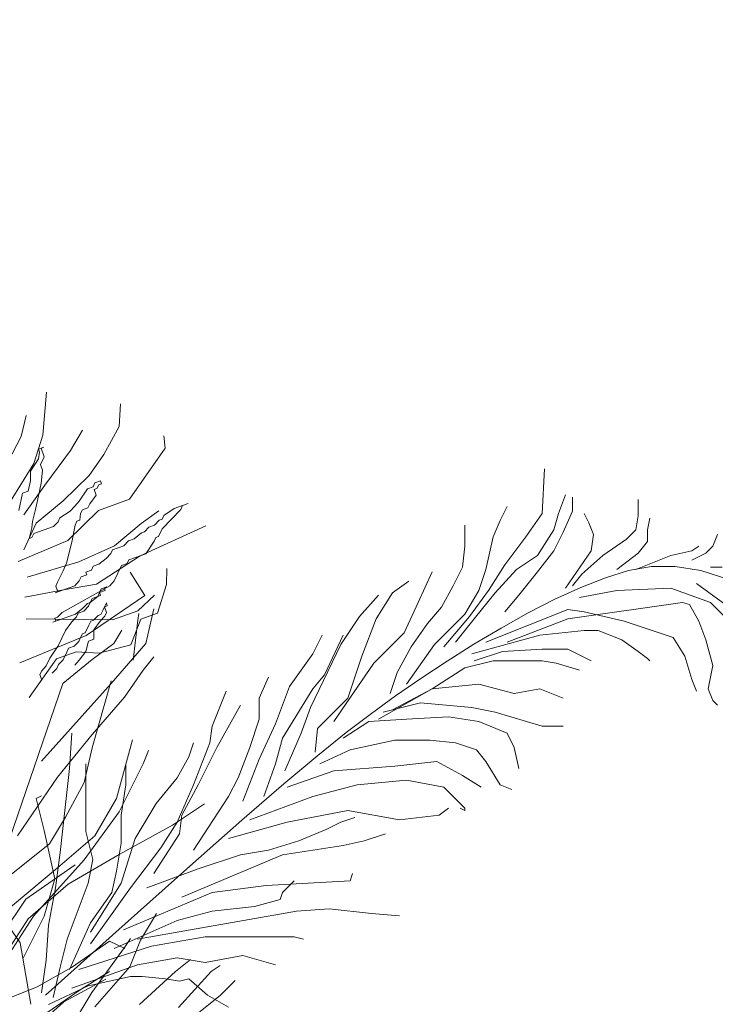
# Model space of a CAD drawing. Units: millimetres. Extents: x 595116 to 630915, y 909473 to 920225.
# Tile 89 of 134: x 629720.901 to 629727.558, y 919275.684 to 919285.103. Entities that reach past the tile are written whole.
import ezdxf

# ---------------------------------------------------------------- set-up
doc = ezdxf.new("R2010")
doc.units = ezdxf.units.MM
doc.layers.add('Dimension', color=3, linetype='Continuous', lineweight=18)
doc.layers.add('L-PLNT', color=85, linetype='Continuous', lineweight=13)
doc.styles.get("Standard").update_dxf_attribs({"font": 'arial.ttf'})
doc.dimstyles.new('ISO-25', dxfattribs={"dimtxt": 9, "dimasz": 6, "dimexe": 1.25, "dimexo": 0.625, "dimtad": 1, "dimlunit": 4, "dimtxsty": 'Standard', "dimcen": 2.5, "dimadec": 0, "dimazin": 0, "dimtfac": 1, "dimtmove": 0, "dimatfit": 3, "dimfxl": 1, "dimarcsym": 0})

# ---------------------------------------------------------------- blocks, each defined once
blk = doc.blocks.new('A$C4FB75ABC')
for p, q in [((2.8876, 3.7608), (2.897, 3.8696)), ((3.0823, 3.7823), (3.0858, 3.8403)), ((2.8322, 3.7571), (2.8454, 3.8105)), ((2.9584, 3.7215), (2.9885, 3.7729)), ((3.043, 3.7114), (3.0823, 3.7823)), ((2.7745, 3.6472), (2.8322, 3.7571)), ((2.8652, 3.6879), (2.8876, 3.7608)), ((3.1994, 3.7272), (3.1962, 3.7584)), ((2.8907, 3.7295), (2.8764, 3.7244)), ((2.8764, 3.7244), (2.8789, 3.7172)), ((2.8789, 3.7172), (2.8769, 3.7003)), ((2.8835, 3.727), (2.8907, 3.7295)), ((2.8913, 3.7054), (2.8835, 3.727)), ((2.893, 3.6331), (2.9584, 3.7215)), ((3.1085, 3.5972), (3.1994, 3.7272)), ((2.8769, 3.7003), (2.856, 3.6684)), ((2.8821, 3.6859), (2.8913, 3.7054)), ((3.0058, 3.6575), (3.043, 3.7114)), ((2.7932, 3.5729), (2.8652, 3.6879)), ((2.856, 3.6684), (2.8566, 3.6443)), ((2.8873, 3.6716), (2.8821, 3.6859)), ((2.8833, 3.6377), (2.8873, 3.6716)), ((4.1608, 3.5609), (4.1668, 3.6742)), ((2.8566, 3.6443), (2.85, 3.6176)), ((2.9398, 3.5932), (3.0058, 3.6575)), ((3.035, 3.6437), (3.0207, 3.6385)), ((3.0376, 3.6365), (3.035, 3.6437)), ((2.85, 3.6176), (2.8356, 3.6125)), ((2.8394, 3.5571), (2.893, 3.6331)), ((2.8746, 3.5941), (2.8833, 3.6377)), ((3.0017, 3.6236), (2.9808, 3.5918)), ((3.0161, 3.6288), (3.0017, 3.6236)), ((3.0207, 3.6385), (3.0161, 3.6288)), ((3.0187, 3.6216), (3.0258, 3.6242)), ((3.0238, 3.6072), (3.0187, 3.6216)), ((3.0258, 3.6242), (3.0304, 3.6339)), ((3.0304, 3.6339), (3.0376, 3.6365)), ((2.8356, 3.6125), (2.827, 3.5688)), ((2.868, 3.5674), (2.8746, 3.5941)), ((2.8712, 3.5361), (2.9398, 3.5932)), ((2.9808, 3.5918), (2.969, 3.5794)), ((3.0075, 3.5852), (3.0238, 3.6072)), ((3.0296, 3.5688), (3.1085, 3.5972)), ((4.2026, 3.5609), (4.2205, 3.6086)), ((4.2384, 3.5668), (4.2384, 3.6026)), ((4.4054, 3.5549), (4.4054, 3.5967)), ((2.8614, 3.5407), (2.868, 3.5674)), ((2.9573, 3.5671), (2.9312, 3.5496)), ((2.9518, 3.4922), (3.0296, 3.5688)), ((2.969, 3.5794), (2.9573, 3.5671)), ((2.984, 3.5605), (2.9885, 3.5702)), ((2.9885, 3.5702), (3.0029, 3.5754)), ((3.0029, 3.5754), (3.0075, 3.5852)), ((3.1389, 3.5352), (3.1839, 3.5676)), ((3.2224, 3.5733), (3.1962, 3.5558)), ((3.2158, 3.5466), (3.2393, 3.5713)), ((3.2582, 3.5862), (3.2224, 3.5733)), ((3.2393, 3.5713), (3.2439, 3.5811)), ((3.2439, 3.5811), (3.2582, 3.5862)), ((4.0535, 3.543), (4.0714, 3.5788)), ((4.2145, 3.5132), (4.2384, 3.5668)), ((2.8594, 3.5238), (2.8614, 3.5407)), ((2.9266, 3.5398), (2.9148, 3.5275)), ((2.9312, 3.5496), (2.9266, 3.5398)), ((2.9702, 3.5312), (2.9748, 3.541)), ((2.9748, 3.541), (2.9819, 3.5435)), ((2.9819, 3.5435), (2.984, 3.5605)), ((3.1845, 3.5435), (3.1727, 3.5311)), ((3.1917, 3.5461), (3.1845, 3.5435)), ((3.1962, 3.5558), (3.1917, 3.5461)), ((3.1922, 3.522), (3.2158, 3.5466)), ((4.0356, 3.5013), (4.0535, 3.543)), ((4.1191, 3.5013), (4.1608, 3.5609)), ((4.1907, 3.5192), (4.2026, 3.5609)), ((4.2801, 3.537), (4.2682, 3.5609)), ((4.3994, 3.5192), (4.4054, 3.5549)), ((4.4293, 3.5192), (4.4352, 3.549)), ((2.8391, 3.4678), (2.8712, 3.5361)), ((2.8528, 3.4971), (2.8594, 3.5238)), ((2.9148, 3.5275), (2.8646, 3.5094)), ((2.9616, 3.4876), (2.9702, 3.5312)), ((3.0703, 3.4781), (3.1389, 3.5352)), ((3.136, 3.4531), (3.303, 3.5294)), ((3.1466, 3.5136), (3.1394, 3.5111)), ((3.1584, 3.526), (3.1466, 3.5136)), ((3.1727, 3.5311), (3.1584, 3.526)), ((3.1831, 3.5024), (3.1922, 3.522)), ((3.964, 3.4774), (3.964, 3.5311)), ((4.1489, 3.4536), (4.1907, 3.5192)), ((4.2921, 3.5072), (4.2801, 3.537)), ((4.3756, 3.4953), (4.3994, 3.5192)), ((4.4293, 3.4893), (4.4293, 3.5192)), ((2.8253, 3.4385), (2.9518, 3.4922)), ((2.86, 3.4997), (2.8528, 3.4971)), ((2.8646, 3.5094), (2.86, 3.4997)), ((3.1062, 3.491), (3.0944, 3.4786)), ((3.1205, 3.4961), (3.1062, 3.491)), ((3.1394, 3.5111), (3.1205, 3.4961)), ((3.1503, 3.4583), (3.1713, 3.4901)), ((3.1713, 3.4901), (3.1759, 3.4999)), ((3.1759, 3.4999), (3.1831, 3.5024)), ((4.0177, 3.4178), (4.0356, 3.5013)), ((4.0654, 3.4297), (4.1191, 3.5013)), ((4.1907, 3.4655), (4.2145, 3.5132)), ((4.2861, 3.4655), (4.2921, 3.5072)), ((4.3159, 3.4536), (4.3756, 3.4953)), ((4.4054, 3.4595), (4.4293, 3.4893)), ((4.5963, 3.4774), (4.6082, 3.5072)), ((2.9484, 3.4342), (2.9616, 3.4876)), ((2.9797, 3.4374), (3.0703, 3.4781)), ((3.0657, 3.4683), (3.0611, 3.4586)), ((3.0944, 3.4786), (3.0657, 3.4683)), ((3.958, 3.4238), (3.964, 3.4774)), ((4.1489, 3.4118), (4.1907, 3.4655)), ((4.2205, 3.3701), (4.2861, 3.4655)), ((4.4889, 3.4536), (4.5426, 3.4655)), ((4.5426, 3.4655), (4.5605, 3.4774)), ((4.5784, 3.4595), (4.5963, 3.4774)), ((3.0244, 3.3805), (3.136, 3.4531)), ((3.0494, 3.4462), (3.0304, 3.4313)), ((3.0611, 3.4586), (3.0494, 3.4462)), ((3.1027, 3.433), (3.1073, 3.4428)), ((3.1073, 3.4428), (3.1503, 3.4583)), ((4.0952, 3.4178), (4.1489, 3.4536)), ((4.2622, 3.4059), (4.3159, 3.4536)), ((4.3517, 3.4178), (4.4054, 3.4595)), ((4.3994, 3.4178), (4.4889, 3.4536)), ((4.5426, 3.4416), (4.5784, 3.4595)), ((2.848, 3.3981), (2.9797, 3.4374)), ((2.9254, 3.3854), (2.9392, 3.4147)), ((2.9392, 3.4147), (2.9484, 3.4342)), ((3.0115, 3.4164), (2.9972, 3.4112)), ((3.0161, 3.4262), (3.0115, 3.4164)), ((3.0304, 3.4313), (3.0161, 3.4262)), ((3.07, 3.3888), (3.0884, 3.4279)), ((3.0884, 3.4279), (3.1027, 3.433)), ((3.2028, 3.3799), (3.2043, 3.4209)), ((3.9342, 3.3761), (3.958, 3.4238)), ((3.9998, 3.3641), (4.0177, 3.4178)), ((4.0237, 3.3641), (4.0654, 3.4297)), ((4.0415, 3.3582), (4.0952, 3.4178)), ((4.322, 3.3969), (4.3813, 3.4152)), ((4.3813, 3.4152), (4.4396, 3.4254)), ((4.4396, 3.4254), (4.5001, 3.426)), ((4.5001, 3.426), (4.5657, 3.4153)), ((4.5657, 3.4153), (4.6395, 3.3917)), ((4.5903, 3.4238), (4.6201, 3.4238)), ((2.9808, 3.3891), (2.969, 3.3768)), ((2.9854, 3.3989), (2.9808, 3.3891)), ((2.9997, 3.4041), (2.9854, 3.3989)), ((2.9972, 3.4112), (2.9997, 3.4041)), ((3.0583, 3.3765), (3.07, 3.3888)), ((3.1481, 3.3521), (3.1105, 3.4115)), ((3.7791, 3.3582), (3.8208, 3.388)), ((3.8447, 3.3343), (3.8805, 3.4118)), ((4.1012, 3.3522), (4.1489, 3.4118)), ((4.2384, 3.3761), (4.2622, 3.4059)), ((4.2593, 3.3722), (4.322, 3.3969)), ((2.8419, 3.3473), (2.9403, 3.3665)), ((2.969, 3.3768), (2.9188, 3.3587)), ((2.9208, 3.3757), (2.9254, 3.3854)), ((2.926, 3.3613), (2.9208, 3.3757)), ((2.9369, 3.3085), (3.0583, 3.3765)), ((2.9403, 3.3665), (3.0244, 3.3805)), ((3.0367, 3.3687), (3.0322, 3.359)), ((3.0322, 3.359), (3.0465, 3.3642)), ((3.0511, 3.3739), (3.0367, 3.3687)), ((3.0439, 3.3713), (3.0511, 3.3739)), ((3.0465, 3.3642), (3.0439, 3.3713)), ((3.1805, 3.307), (3.2028, 3.3799)), ((3.9044, 3.3224), (3.9342, 3.3761)), ((3.964, 3.3045), (3.9998, 3.3641)), ((3.9759, 3.2986), (4.0237, 3.3641)), ((4.1935, 3.342), (4.2593, 3.3722)), ((4.2563, 3.3463), (4.3517, 3.3641)), ((4.3517, 3.3641), (4.4889, 3.3701)), ((4.4889, 3.3701), (4.5903, 3.3343)), ((4.5545, 3.382), (4.6858, 3.2866)), ((2.9188, 3.3587), (2.926, 3.3613)), ((2.9986, 3.2497), (3.1481, 3.3521)), ((3.0276, 3.3492), (3.0086, 3.3343)), ((3.0086, 3.3343), (3.0132, 3.3441)), ((3.0132, 3.3441), (3.0347, 3.3518)), ((3.0322, 3.359), (3.0276, 3.3492)), ((3.0347, 3.3518), (3.0322, 3.359)), ((3.1297, 3.313), (3.1722, 3.3526)), ((3.6956, 3.2986), (3.7433, 3.3522)), ((3.7373, 3.2926), (3.7791, 3.3582)), ((3.9879, 3.2926), (4.0415, 3.3582)), ((4.0654, 3.3105), (4.1012, 3.3522)), ((4.1256, 3.3072), (4.1935, 3.342)), ((2.9897, 3.3194), (2.9708, 3.3045)), ((3.0015, 3.3317), (2.9897, 3.3194)), ((2.9923, 3.3122), (3.004, 3.3246)), ((3.0086, 3.3343), (3.0015, 3.3317)), ((3.004, 3.3246), (3.0086, 3.3343)), ((3.0359, 3.3036), (3.0405, 3.3134)), ((3.0405, 3.3134), (3.0451, 3.3231)), ((3.0497, 3.3329), (3.0451, 3.3231)), ((3.0451, 3.3231), (3.0522, 3.3257)), ((3.0451, 3.3231), (3.0502, 3.3088)), ((3.0522, 3.3257), (3.0497, 3.3329)), ((3.0651, 3.2898), (3.1297, 3.313)), ((3.1501, 3.2292), (3.1706, 3.3178)), ((3.8089, 3.2568), (3.8447, 3.3343)), ((3.8686, 3.2807), (3.9044, 3.3224)), ((4.0177, 3.233), (4.2265, 3.3164)), ((4.2265, 3.2926), (4.5187, 3.3343)), ((4.2265, 3.3164), (4.2682, 3.3105)), ((4.5187, 3.3343), (4.5366, 3.3284)), ((4.5366, 3.3284), (4.5605, 3.2866)), ((4.5903, 3.3343), (4.644, 3.2807)), ((2.8457, 3.2919), (3.0651, 3.2898)), ((2.9708, 3.3045), (2.9134, 3.2838)), ((2.918, 3.2936), (2.9251, 3.2962)), ((2.9206, 3.2864), (2.918, 3.2936)), ((2.9251, 3.2962), (2.9369, 3.3085)), ((2.9616, 3.285), (2.9733, 3.2973)), ((2.9733, 3.2973), (2.9779, 3.3071)), ((2.9779, 3.3071), (2.9923, 3.3122)), ((3.0098, 3.2861), (3.0169, 3.2887)), ((3.0169, 3.2887), (3.0287, 3.301)), ((3.0287, 3.301), (3.0359, 3.3036)), ((3.0456, 3.299), (3.0339, 3.2867)), ((3.0502, 3.3088), (3.0456, 3.299)), ((3.1125, 3.2258), (3.1374, 3.2915)), ((3.1182, 3.1873), (3.1303, 3.2889)), ((3.1303, 3.2889), (3.1323, 3.3059)), ((3.1374, 3.2915), (3.1805, 3.307)), ((3.6479, 3.227), (3.6956, 3.2986)), ((3.7015, 3.1972), (3.7373, 3.2926)), ((3.8865, 3.227), (3.964, 3.3045)), ((3.9103, 3.2211), (3.9759, 3.2986)), ((3.9401, 3.233), (3.9879, 3.2926)), ((4.0565, 3.2687), (4.1256, 3.3072)), ((4.0714, 3.233), (4.2265, 3.2926)), ((4.2682, 3.3105), (4.3696, 3.2866)), ((2.9134, 3.2838), (2.9206, 3.2864)), ((2.936, 3.2434), (2.9452, 3.2629)), ((2.9452, 3.2629), (2.9616, 3.285)), ((2.996, 3.2568), (3.0052, 3.2763)), ((3.0052, 3.2763), (3.0098, 3.2861)), ((3.0339, 3.2867), (3.0175, 3.2646)), ((3.0175, 3.2646), (3.0181, 3.2405)), ((3.0684, 3.2292), (3.0888, 3.2633)), ((3.8268, 3.2211), (3.8686, 3.2807)), ((3.9871, 3.2274), (4.0565, 3.2687)), ((4.1549, 3.2509), (4.2682, 3.2628)), ((4.2682, 3.2628), (4.304, 3.2628)), ((4.304, 3.2628), (4.3637, 3.2389)), ((4.3696, 3.2866), (4.4412, 3.2628)), ((4.4412, 3.2628), (4.4949, 3.2449)), ((4.5605, 3.2866), (4.5784, 3.2389)), ((2.829, 3.1805), (2.9986, 3.2497)), ((2.9269, 3.2238), (2.936, 3.2434)), ((2.9797, 3.2347), (2.9842, 3.2445)), ((2.9842, 3.2445), (2.9888, 3.2542)), ((2.9888, 3.2542), (2.996, 3.2568)), ((3.0181, 3.2405), (3.0038, 3.2353)), ((3.5763, 3.2032), (3.6001, 3.2509)), ((3.6061, 3.1495), (3.6538, 3.2509)), ((3.7314, 3.1793), (3.8089, 3.2568)), ((3.9819, 3.2032), (4.1549, 3.2509)), ((4.3637, 3.2389), (4.4054, 3.2091)), ((4.4949, 3.2449), (4.5247, 3.1972)), ((4.5784, 3.2389), (4.5963, 3.1734)), ((2.9059, 3.192), (2.9269, 3.2238)), ((2.949, 3.2075), (2.9535, 3.2172)), ((2.9535, 3.2172), (2.9679, 3.2224)), ((2.9679, 3.2224), (2.9797, 3.2347)), ((3.0038, 3.2353), (2.9972, 3.2086)), ((3.0139, 3.1884), (3.0684, 3.2292)), ((3.031, 3.2046), (3.1125, 3.2258)), ((3.0616, 3.1271), (3.1501, 3.2292)), ((3.5703, 3.066), (3.6479, 3.227)), ((3.791, 3.1555), (3.8268, 3.2211)), ((3.8149, 3.1257), (3.8865, 3.227)), ((3.9185, 3.1843), (3.9871, 3.2274)), ((4.0594, 3.2091), (4.1608, 3.2151)), ((4.1608, 3.2151), (4.2265, 3.2151)), ((4.2265, 3.2151), (4.2861, 3.1853)), ((2.8529, 3.0918), (2.9229, 3.19)), ((2.8967, 3.1725), (2.9059, 3.192)), ((2.9229, 3.19), (2.9731, 3.208)), ((2.928, 3.1756), (2.9398, 3.188)), ((2.9389, 3.1271), (3.0139, 3.1884)), ((2.9398, 3.188), (2.949, 3.2075)), ((2.9731, 3.208), (3.031, 3.2046)), ((2.9972, 3.2086), (2.9808, 3.1865)), ((3.1433, 3.1611), (3.1706, 3.1952)), ((3.5166, 3.1197), (3.5763, 3.2032)), ((3.6658, 3.0899), (3.7015, 3.1972)), ((3.9879, 3.1853), (4.0594, 3.2091)), ((4.4054, 3.2091), (4.4293, 3.1912)), ((4.4293, 3.1912), (4.4352, 3.1853)), ((4.5247, 3.1972), (4.5426, 3.1376)), ((2.885, 3.1601), (2.8967, 3.1725)), ((2.9117, 3.1535), (2.9234, 3.1659)), ((2.9234, 3.1659), (2.928, 3.1756)), ((2.9808, 3.1865), (2.969, 3.1742)), ((3.63, 3.0303), (3.7314, 3.1793)), ((3.8516, 3.1401), (3.9185, 3.1843)), ((3.8805, 3.1137), (3.964, 3.1674)), ((3.964, 3.1674), (4.0356, 3.1853)), ((4.0356, 3.1853), (4.1072, 3.1853)), ((4.1072, 3.1853), (4.1608, 3.1853)), ((4.1608, 3.1853), (4.1966, 3.1793)), ((4.1966, 3.1793), (4.2563, 3.1614)), ((4.5963, 3.1734), (4.5844, 3.1137)), ((2.8804, 3.1504), (2.885, 3.1601)), ((2.8856, 3.136), (2.8804, 3.1504)), ((3.0956, 3.093), (3.1433, 3.1611)), ((3.4391, 3.0899), (3.4629, 3.1436)), ((3.5763, 3.1137), (3.6061, 3.1495)), ((3.7731, 3.1018), (3.791, 3.1555)), ((3.7873, 3.0958), (3.8516, 3.1401)), ((4.5426, 3.1376), (4.5545, 3.1078)), ((2.7823, 2.6709), (2.9389, 3.1271)), ((2.8844, 2.9296), (3.0616, 3.1271)), ((3.0139, 2.9637), (3.0616, 3.1339)), ((3.4808, 3.0243), (3.5166, 3.1197)), ((3.4987, 2.9885), (3.5763, 3.1137)), ((3.7433, 3.0362), (3.8805, 3.1137)), ((3.7791, 3.0601), (3.8805, 3.1137)), ((3.8805, 3.1137), (3.9998, 3.1257)), ((3.9998, 3.1257), (4.0893, 3.1018)), ((4.0893, 3.1018), (4.1549, 3.1137)), ((4.1549, 3.1137), (4.2145, 3.0899)), ((4.5844, 3.1137), (4.5963, 3.0839)), ((3.0139, 2.9977), (3.0956, 3.093)), ((3.3198, 3.0184), (3.3556, 3.1078)), ((3.4391, 3.0362), (3.4391, 3.0899)), ((3.5882, 3.0124), (3.6658, 3.0899)), ((3.7254, 3.0513), (3.7873, 3.0958)), ((3.3317, 2.9647), (3.3914, 3.072)), ((3.5465, 3.0005), (3.5703, 3.066)), ((3.7552, 3.0541), (3.8507, 3.078)), ((3.8507, 3.078), (3.9819, 3.066)), ((3.9819, 3.066), (4.0415, 3.0541)), ((4.5963, 3.0839), (4.6082, 3.072)), ((3.6611, 3.0024), (3.7254, 3.0513)), ((3.8149, 3.0362), (3.9222, 3.0422)), ((3.9222, 3.0422), (3.9998, 3.0303)), ((4.0415, 3.0541), (4.1608, 3.0184)), ((3.3138, 2.9766), (3.3198, 3.0184)), ((3.4152, 2.9647), (3.4391, 3.0362)), ((3.4391, 2.9349), (3.4808, 3.0243)), ((3.5822, 2.9528), (3.5882, 3.0124)), ((3.6538, 2.9885), (3.7194, 3.0303)), ((3.7194, 3.0303), (3.8149, 3.0362)), ((3.9998, 3.0303), (4.0714, 3.0005)), ((4.1608, 3.0184), (4.2145, 3.0184)), ((2.9253, 2.8888), (3.0139, 2.9977)), ((2.9559, 2.911), (2.9619, 3.0005)), ((3.4808, 2.923), (3.4987, 2.9885)), ((3.5047, 2.9051), (3.5465, 3.0005)), ((3.5886, 2.9442), (3.6611, 3.0024)), ((4.0714, 3.0005), (4.0893, 2.9647)), ((2.9935, 2.8751), (3.0139, 2.9637)), ((3.0752, 2.8343), (3.1161, 2.9841)), ((3.2601, 2.9408), (3.2721, 2.9766)), ((3.2721, 2.8693), (3.3138, 2.9766)), ((3.284, 2.8693), (3.3317, 2.9647)), ((3.3854, 2.8872), (3.4152, 2.9647)), ((3.6717, 2.9587), (3.7851, 2.9826)), ((3.7851, 2.9826), (3.8745, 2.9826)), ((3.8745, 2.9826), (3.9401, 2.9766)), ((3.9401, 2.9766), (3.9938, 2.9587)), ((4.0893, 2.9647), (4.1012, 2.911)), ((3.1433, 2.9228), (3.157, 2.9569)), ((3.2303, 2.8872), (3.2601, 2.9408)), ((3.5019, 2.8714), (3.5886, 2.9442)), ((3.5942, 2.923), (3.6717, 2.9587)), ((3.9938, 2.9587), (4.0177, 2.9289)), ((2.9977, 2.8216), (2.9977, 2.923)), ((3.082, 2.8002), (3.1433, 2.9228)), ((3.0991, 2.8693), (3.0991, 2.923)), ((3.3973, 2.8276), (3.4391, 2.9349)), ((3.451, 2.8395), (3.4808, 2.923)), ((3.63, 2.9051), (3.7851, 2.917)), ((3.7851, 2.917), (3.8924, 2.9289)), ((3.8924, 2.9289), (3.958, 2.8932)), ((4.0177, 2.9289), (4.0535, 2.8693)), ((2.8231, 2.739), (2.9253, 2.8888)), ((2.944, 2.8037), (2.9559, 2.911)), ((3.1766, 2.8216), (3.2303, 2.8872)), ((3.3615, 2.8395), (3.3854, 2.8872)), ((3.5107, 2.8633), (3.63, 2.9051)), ((3.958, 2.8932), (4.0058, 2.8633)), ((2.9458, 2.7866), (2.9935, 2.8751)), ((3.0872, 2.7918), (3.0991, 2.8693)), ((3.2303, 2.7739), (3.2721, 2.8693)), ((3.2422, 2.7918), (3.284, 2.8693)), ((3.3951, 2.779), (3.5019, 2.8714)), ((3.5763, 2.8395), (3.6896, 2.8693)), ((3.6896, 2.8693), (3.8149, 2.8812)), ((3.8149, 2.8812), (3.9103, 2.8633)), ((3.9103, 2.8633), (3.964, 2.8097)), ((4.0535, 2.8693), (4.0833, 2.8574)), ((2.8708, 2.8343), (2.8844, 2.8411)), ((3.2721, 2.7024), (3.3615, 2.8395)), ((3.4152, 2.7799), (3.5763, 2.8395)), ((2.8913, 2.7526), (2.8708, 2.8343)), ((2.9977, 2.7501), (2.9977, 2.8216)), ((3.0207, 2.739), (3.0752, 2.8343)), ((3.1229, 2.7322), (3.1766, 2.8216)), ((3.2183, 2.7662), (3.3, 2.8207)), ((2.9049, 2.7185), (2.9458, 2.7866)), ((2.9321, 2.6964), (2.944, 2.8037)), ((2.9935, 2.6777), (3.082, 2.8002)), ((3.0872, 2.7203), (3.0872, 2.7918)), ((3.2363, 2.7441), (3.2422, 2.7918)), ((3.5107, 2.7739), (3.6658, 2.8037)), ((3.6479, 2.7739), (3.6837, 2.7858)), ((3.6658, 2.8037), (3.797, 2.7799)), ((3.797, 2.7799), (3.8984, 2.7918)), ((3.8984, 2.7918), (3.9222, 2.8097)), ((3.964, 2.8037), (3.9521, 2.8097)), ((3.964, 2.8097), (3.964, 2.8037)), ((3.082, 2.6913), (3.2183, 2.7662)), ((3.1886, 2.7083), (3.2303, 2.7739)), ((3.2623, 2.6619), (3.3951, 2.779)), ((3.3615, 2.7322), (3.5107, 2.7739)), ((3.6121, 2.756), (3.6479, 2.7739)), ((2.9185, 2.63), (2.8913, 2.7526)), ((2.9253, 2.6572), (3.0207, 2.739)), ((3.0156, 2.6785), (2.9977, 2.7501)), ((3.1707, 2.6428), (3.2363, 2.7441)), ((3.5405, 2.7262), (3.6121, 2.756)), ((3.7075, 2.7262), (3.7612, 2.7441)), ((2.7414, 2.5891), (2.9049, 2.7185)), ((3.0752, 2.6487), (3.0872, 2.7203)), ((3.0872, 2.6189), (3.1229, 2.7322)), ((3.4629, 2.7024), (3.5405, 2.7262)), ((3.4987, 2.6904), (3.6538, 2.7143)), ((3.6538, 2.7143), (3.7075, 2.7262)), ((2.9201, 2.607), (2.9321, 2.6964)), ((2.9526, 2.6164), (3.082, 2.6913)), ((3.111, 2.607), (3.1886, 2.7083)), ((3.2422, 2.5831), (3.4987, 2.6904)), ((3.284, 2.6547), (3.3914, 2.6904)), ((3.3914, 2.6904), (3.4629, 2.7024)), ((2.8442, 2.5778), (2.9704, 2.6651)), ((2.864, 2.5347), (2.9935, 2.6777)), ((3.0036, 2.6189), (3.0156, 2.6785)), ((3.0976, 2.5149), (3.2623, 2.6619)), ((2.7209, 2.487), (2.9253, 2.6572)), ((3.0633, 2.5951), (3.0752, 2.6487)), ((3.1528, 2.607), (3.284, 2.6547)), ((3.6717, 2.6249), (3.6777, 2.6428)), ((2.8504, 2.5279), (2.9526, 2.6164)), ((2.8913, 2.5347), (2.9185, 2.63)), ((2.95, 2.4758), (3.0036, 2.6189)), ((3.0096, 2.4937), (3.0872, 2.6189)), ((3.3198, 2.5951), (3.457, 2.6129)), ((3.457, 2.6129), (3.6717, 2.6249)), ((3.4987, 2.5951), (3.5286, 2.6249)), ((2.9022, 2.5116), (2.9201, 2.607)), ((3.0096, 2.4639), (3.111, 2.607)), ((3.0096, 2.5176), (3.0633, 2.5951)), ((3.0931, 2.4997), (3.3198, 2.5951)), ((3.4928, 2.5772), (3.4987, 2.5951)), ((2.786, 2.4905), (2.8442, 2.5778)), ((3.4272, 2.5593), (3.4928, 2.5772)), ((2.8299, 2.4666), (2.7686, 2.5551)), ((3.1289, 2.4758), (3.5345, 2.5474)), ((3.1365, 2.4734), (3.1774, 2.5415)), ((3.2303, 2.5235), (3.3198, 2.5474)), ((3.3198, 2.5474), (3.4272, 2.5593)), ((3.5345, 2.5474), (3.618, 2.5533)), ((3.618, 2.5533), (3.7254, 2.5414)), ((3.7254, 2.5414), (3.797, 2.5354)), ((2.7891, 2.4325), (2.8504, 2.5279)), ((2.8027, 2.4393), (2.864, 2.5347)), ((2.8368, 2.4257), (2.8913, 2.5347)), ((2.895, 2.333), (3.0976, 2.5149)), ((2.8963, 2.4222), (2.9022, 2.5116)), ((2.9559, 2.3983), (3.0096, 2.5176)), ((3.0693, 2.452), (3.2303, 2.5235)), ((2.8572, 2.31), (2.8299, 2.4666)), ((2.9321, 2.4043), (2.95, 2.4758)), ((2.9607, 2.4032), (3.0578, 2.4711)), ((3.0578, 2.4711), (3.0966, 2.4517)), ((3.0962, 2.4544), (3.1115, 2.4773)), ((3.1093, 2.4053), (3.1365, 2.4734)), ((3.1647, 2.4579), (3.3019, 2.4818)), ((3.3019, 2.4818), (3.4152, 2.4818)), ((3.4152, 2.4818), (3.5286, 2.4818)), ((3.5286, 2.4818), (3.5524, 2.4758)), ((2.9798, 2.3983), (3.1647, 2.4579)), ((3.0123, 2.3401), (3.0962, 2.4544)), ((2.8844, 2.3387), (2.8963, 2.4222)), ((2.9619, 2.3506), (3.1289, 2.4102)), ((3.1289, 2.4102), (3.2303, 2.4281)), ((3.2259, 2.3934), (3.264, 2.4239)), ((3.2303, 2.4281), (3.3019, 2.4162)), ((3.3019, 2.4162), (3.3973, 2.4341)), ((3.3973, 2.4341), (3.4808, 2.4102)), ((2.8733, 2.3546), (2.9607, 2.4032)), ((2.9142, 2.3268), (2.9321, 2.4043)), ((2.9801, 2.3449), (3.0578, 2.3935)), ((3.0207, 2.3031), (3.1093, 2.4053)), ((3.1344, 2.3096), (3.2259, 2.3934)), ((3.2335, 2.302), (3.3174, 2.3934)), ((3.3174, 2.3934), (3.3403, 2.4087)), ((2.9413, 2.3158), (3.0481, 2.3741)), ((3.0036, 2.3566), (3.111, 2.3804)), ((3.111, 2.3804), (3.1408, 2.3804)), ((3.1408, 2.3804), (3.2005, 2.3745)), ((3.2005, 2.3745), (3.2363, 2.3685)), ((3.2363, 2.3685), (3.2601, 2.3745)), ((3.2601, 2.3745), (3.3079, 2.3327)), ((3.3403, 2.3324), (3.3784, 2.3706)), ((2.7277, 2.2964), (2.8733, 2.3546)), ((2.8539, 2.2576), (2.9801, 2.3449)), ((2.9022, 2.3089), (3.0036, 2.3566)), ((2.9666, 2.2638), (3.0123, 2.3401)), ((2.8539, 2.2382), (2.9413, 2.3158)), ((3.264, 2.2715), (3.3403, 2.3324)), ((3.3079, 2.3327), (3.3615, 2.3029))]:
    blk.add_line(p, q)
blk = doc.blocks.new('*D216')
at = {"layer": 'Defpoints', "color": 0, "transparency": 16777216}
for p in [(629743.5408, 919411.9276), (629505.0408, 919411.8279), (629743.5408, 918832.3776)]:
    blk.add_point(p, dxfattribs=at)
at = {"layer": 'Dimension', "color": 0, "lineweight": -2, "transparency": 16777216}
for p, q in [((629743.5408, 919411.3026), (629743.5408, 918831.1276)), ((629505.0408, 919411.2029), (629505.0408, 918831.1276)), ((629511.0408, 918832.3776), (629737.5408, 918832.3776))]:
    blk.add_line(p, q, dxfattribs=at)
at = {"layer": 'Dimension', "color": 0, "transparency": 16777216}
for points in [[(629511.0408, 918833.3776), (629511.0408, 918831.3776), (629505.0408, 918832.3776)], [(629737.5408, 918833.3776), (629737.5408, 918831.3776), (629743.5408, 918832.3776)]]:
    blk.add_solid(points, dxfattribs=at)
at = {"layer": 'Dimension', "color": 0, "transparency": 16777216, "insert": (629624.2908, 918837.656), "char_height": 9, "attachment_point": 5}
blk.add_mtext('19\'-10 1/2"', dxfattribs=at)

msp = doc.modelspace()

# ---------------------------------------------------------------- block references
at = {"layer": 'L-PLNT', "xscale": 3.753413438031968, "yscale": 3.753413438031968, "zscale": 3.753413438031968}
msp.add_blockref('A$C4FB75ABC', (629710.2837, 919267.0144), dxfattribs=at)

# ---------------------------------------------------------------- dimensions: what is measured, and where the dimension line sits
at = {"layer": 'Dimension'}
dim = msp.add_linear_dim(base=(629743.5408, 918832.3776), p1=(629505.0408, 919411.8279), p2=(629743.5408, 919411.9276), dimstyle='ISO-25', override={"dimdec": 1, "dimlfac": 1, "dimrnd": 0, "dimzin": 1, "dimdsep": 46, "dimlunit": 4, "dimfrac": 2}, dxfattribs=at)
dim.commit()
dim.dimension.update_dxf_attribs({"geometry": '*D216', "text_midpoint": (629624.2908, 918837.656)})

doc.saveas('drawing.dxf')
